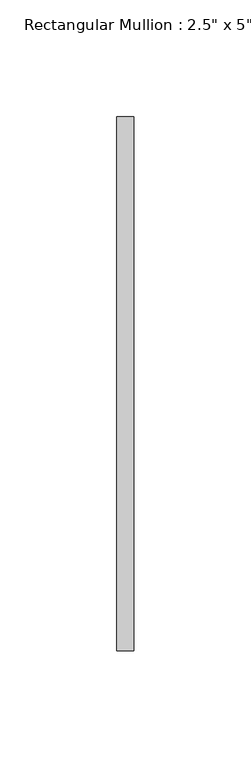
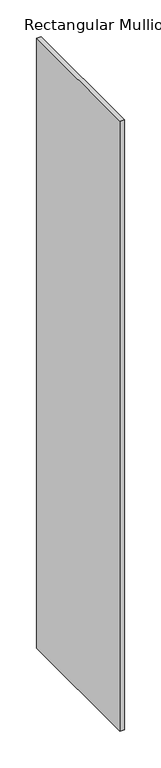
"""IFC4 building model written with IfcOpenShell, lengths in millimetres: member geometry."""

from ifc_helpers import new_model, si_unit, frame, origin, place, context, project, spatial, polyline, outline, extrude, source, transform, mapped, element, save


def member_1d4720dc(model_context):
    return source(origin(), model_context, "Body", "SweptSolid", [
        extrude(outline(polyline([(3.6195, 114.3), (3.6195, -114.3), (-3.6195, -114.3), (-3.6195, 114.3), (3.6195, 114.3)])), frame((0.0, 0.0, -1017.8415), z_axis=(0.0, 0.0, 1.0), x_axis=(1.0, 0.0, 0.0)), (0.0, 0.0, 1.0), 1017.8415),
    ])


if __name__ == "__main__":
    model = new_model("IFC4")
    model_context = context("Model", 3, world=origin())
    ifc_project = project(units=[si_unit("LENGTHUNIT", "METRE", prefix="MILLI")], contexts=[model_context])
    site = spatial("IfcSite", under=ifc_project)
    building = spatial("IfcBuilding", under=site)
    placement = place(None, origin())
    member_shape = member_1d4720dc(model_context)
    element("IfcMember", 1, ObjectType="Rectangular Mullion : 2.5\" x 5\" rectangular", at=placement, inside=building, context=model_context, shape_type="MappedRepresentation", body=[
        mapped(member_shape, transform((0.0, 0.0, 0.0), x_axis=(1.0, 0.0, 0.0), y_axis=(0.0, 1.0, 0.0), z_axis=(0.0, 0.0, 1.0))),
    ])
    save(model, "model.ifc")

# Revit data of these elements
# Type "Rectangular Mullion : 2.5\" x 5\" rectangular"
#   built-in parameter 1007304 = 0.75 (stored number, unit not read)
#   built-in parameter 1007301 = 0.011875 (stored number, unit not read)
#   built-in parameter 1007300 = 0.011875 (stored number, unit not read)
# Element 1 (IfcMember, "Rectangular Mullion : 2.5\" x 5\" rectangular")
#   Materials on its faces: "WINDOW GLASS MATERIAL"
# Materials
#   "WINDOW GLASS MATERIAL": class "Generic", colour RGB 120 120 120, transparency 0, Cost = 0
